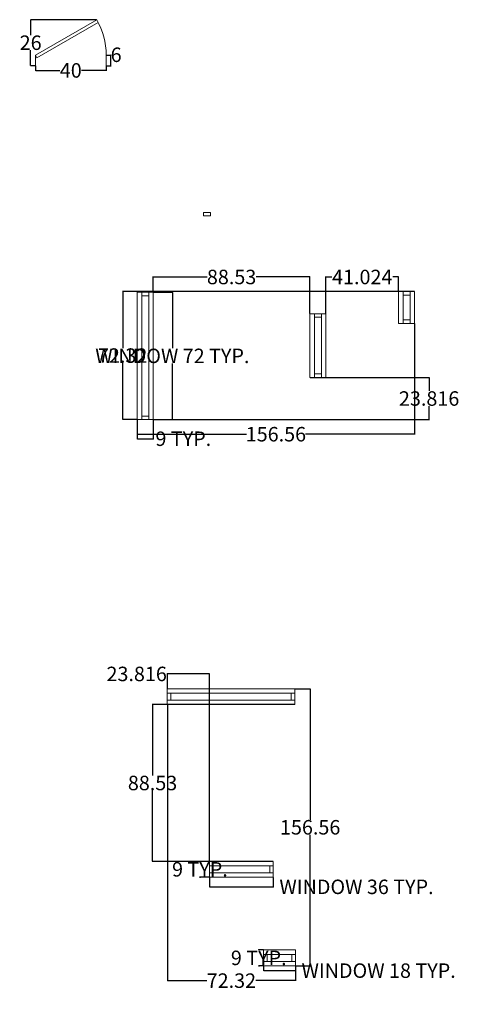
# Model space of a CAD drawing. Units: inches. Extents: x -254 to 1961, y 86 to 3025.
# Tile 4 of 6: x 580 to 828, y 86 to 642. Entities that reach past the tile are written whole.
import ezdxf

# ---------------------------------------------------------------- set-up
doc = ezdxf.new("R2010")
doc.units = ezdxf.units.IN
doc.header["$MEASUREMENT"] = 0
for name, color, linetype, lineweight in [('A-ANNO-DIMS', 2, 'Continuous', 18), ('DOORS', 40, 'Continuous', 18), ('WINDOWS', 50, 'Continuous', 18)]:
    doc.layers.add(name, color=color, linetype=linetype, lineweight=lineweight)
doc.styles.get("Standard").update_dxf_attribs({"font": 'arial.ttf'})
doc.dimstyles.get("Standard").update_dxf_attribs({"dimtxt": 8.18, "dimasz": 0.18, "dimexe": 0.18, "dimexo": 0.0625, "dimgap": 0.09, "dimtad": 0, "dimtih": 1, "dimtoh": 1, "dimdec": 1, "dimzin": 0, "dimdsep": 46, "dimlunit": 3, "dimtxsty": 'Standard', "dimcen": 0.09, "dimadec": 0, "dimazin": 0, "dimtfac": 1, "dimtdec": 1, "dimtofl": 0, "dimtmove": 0, "dimatfit": 3, "dimfxl": 1, "dimtolj": 1, "dimtzin": 0, "dimarcsym": 0})

# ---------------------------------------------------------------- blocks, each defined once
blk = doc.blocks.new('*U2')
for p, q in [((0, 0), (0, -6)), ((40, 0), (40, -6))]:
    blk.add_line(p, q)
blk.add_lwpolyline([(0, 0), (34.64, 20), (35.52, 18.48), (0.87, -1.52)], close=True)
blk.add_arc((0, 0), 40, 0, 30)
blk = doc.blocks.new('WIN-36IN')
for p, q in [((2.5, 35), (2.5, 2)), ((6.5, 35), (6.5, 2))]:
    blk.add_line(p, q)
for points in [[(0, 36), (9, 36), (9, 0), (0, 0)], [(2.5, 36), (6.5, 36), (6.5, 34), (2.5, 34)], [(2.5, 0), (6.5, 0), (6.5, 2), (2.5, 2)]]:
    blk.add_lwpolyline(points, close=True)
blk = doc.blocks.new('WIN-72IN')
for p, q in [((2.5, 70), (2.5, 2)), ((6.5, 70), (6.5, 2))]:
    blk.add_line(p, q)
for points in [[(0, 72), (9, 72), (9, 0), (0, 0)], [(2.5, 72), (6.5, 72), (6.5, 70), (2.5, 70)], [(2.5, 0), (6.5, 0), (6.5, 2), (2.5, 2)]]:
    blk.add_lwpolyline(points, close=True)
blk = doc.blocks.new('WIN-18IN')
for p, q in [((2.5, 16), (2.5, 2)), ((6.5, 16), (6.5, 2))]:
    blk.add_line(p, q)
for points in [[(0, 18), (9, 18), (9, 0), (0, 0)], [(2.5, 18), (6.5, 18), (6.5, 16), (2.5, 16)], [(2.5, 0), (6.5, 0), (6.5, 2), (2.5, 2)]]:
    blk.add_lwpolyline(points, close=True)
blk = doc.blocks.new('*D14')
at = {"layer": 'A-ANNO-DIMS', "color": 0, "lineweight": -2, "transparency": 16777216}
for p, q in [((655.23, 487.85), (666.15, 487.85)), ((665.97, 487.67), (665.97, 456.17)), ((665.97, 416.03), (665.97, 447.53)), ((655.23, 415.85), (666.15, 415.85))]:
    blk.add_line(p, q, dxfattribs=at)
at = {"layer": 'A-ANNO-DIMS', "color": 0, "transparency": 16777216}
for points in [[(665.94, 487.67), (666, 487.67), (665.97, 487.85)], [(665.94, 416.03), (666, 416.03), (665.97, 415.85)]]:
    blk.add_solid(points, dxfattribs=at)
at = {"layer": 'Defpoints', "color": 0, "transparency": 16777216}
for p in [(655.17, 487.85), (665.97, 487.85), (655.17, 415.85)]:
    blk.add_point(p, dxfattribs=at)
at = {"layer": 'A-ANNO-DIMS', "color": 0, "transparency": 16777216, "insert": (665.97, 451.85), "char_height": 8.18, "attachment_point": 5}
blk.add_mtext('\\A1;WINDOW 72 TYP.', dxfattribs=at)
blk = doc.blocks.new('*D15')
at = {"layer": 'A-ANNO-DIMS', "color": 0, "lineweight": -2, "transparency": 16777216}
for p, q in [((646.17, 415.79), (646.17, 404.87)), ((655.17, 415.79), (655.17, 404.87)), ((646.35, 405.05), (654.99, 405.05)), ((655.17, 405.05), (655.35, 405.05))]:
    blk.add_line(p, q, dxfattribs=at)
at = {"layer": 'A-ANNO-DIMS', "color": 0, "transparency": 16777216}
for points in [[(646.35, 405.08), (646.35, 405.02), (646.17, 405.05)], [(654.99, 405.08), (654.99, 405.02), (655.17, 405.05)]]:
    blk.add_solid(points, dxfattribs=at)
at = {"layer": 'Defpoints', "color": 0, "transparency": 16777216}
for p in [(646.17, 415.85), (655.17, 415.85), (655.17, 405.05)]:
    blk.add_point(p, dxfattribs=at)
at = {"layer": 'A-ANNO-DIMS', "color": 0, "transparency": 16777216, "insert": (672.17, 405.05), "char_height": 8.18, "attachment_point": 5}
blk.add_mtext('\\A1;9 TYP.', dxfattribs=at)
blk = doc.blocks.new('*D16')
at = {"layer": 'A-ANNO-DIMS', "color": 0, "lineweight": -2, "transparency": 16777216}
for p, q in [((686.95, 157.24), (686.95, 151.73)), ((722.95, 157.24), (722.95, 151.73)), ((687.13, 151.91), (722.77, 151.91)), ((722.95, 151.91), (723.13, 151.91))]:
    blk.add_line(p, q, dxfattribs=at)
at = {"layer": 'A-ANNO-DIMS', "color": 0, "transparency": 16777216}
for points in [[(687.13, 151.94), (687.13, 151.88), (686.95, 151.91)], [(722.77, 151.94), (722.77, 151.88), (722.95, 151.91)]]:
    blk.add_solid(points, dxfattribs=at)
at = {"layer": 'Defpoints', "color": 0, "transparency": 16777216}
for p in [(686.95, 157.31), (722.95, 157.31), (722.95, 151.91)]:
    blk.add_point(p, dxfattribs=at)
at = {"layer": 'A-ANNO-DIMS', "color": 0, "transparency": 16777216, "insert": (769.96, 151.91), "char_height": 8.18, "attachment_point": 5}
blk.add_mtext('\\A1;WINDOW 36 TYP.', dxfattribs=at)
blk = doc.blocks.new('*D17')
at = {"layer": 'A-ANNO-DIMS', "color": 0, "lineweight": -2, "transparency": 16777216}
for p, q in [((686.89, 166.31), (681.37, 166.31)), ((681.55, 166.49), (681.55, 166.67)), ((686.89, 157.31), (681.37, 157.31)), ((681.55, 157.13), (681.55, 156.95))]:
    blk.add_line(p, q, dxfattribs=at)
at = {"layer": 'A-ANNO-DIMS', "color": 0, "transparency": 16777216}
for points in [[(681.52, 166.49), (681.58, 166.49), (681.55, 166.31)], [(681.52, 157.13), (681.58, 157.13), (681.55, 157.31)]]:
    blk.add_solid(points, dxfattribs=at)
at = {"layer": 'Defpoints', "color": 0, "transparency": 16777216}
for p in [(686.95, 166.31), (681.55, 157.31), (686.95, 157.31)]:
    blk.add_point(p, dxfattribs=at)
at = {"layer": 'A-ANNO-DIMS', "color": 0, "transparency": 16777216, "insert": (681.55, 161.81), "char_height": 8.18, "attachment_point": 5}
blk.add_mtext('\\A1;9 TYP.', dxfattribs=at)
blk = doc.blocks.new('*D18')
at = {"layer": 'A-ANNO-DIMS', "color": 0, "lineweight": -2, "transparency": 16777216}
for p, q in [((717.45, 107.22), (717.45, 104.4)), ((735.45, 107.22), (735.45, 104.4)), ((717.63, 104.58), (735.27, 104.58)), ((735.45, 104.58), (735.63, 104.58))]:
    blk.add_line(p, q, dxfattribs=at)
at = {"layer": 'A-ANNO-DIMS', "color": 0, "transparency": 16777216}
for points in [[(717.63, 104.61), (717.63, 104.55), (717.45, 104.58)], [(735.27, 104.61), (735.27, 104.55), (735.45, 104.58)]]:
    blk.add_solid(points, dxfattribs=at)
at = {"layer": 'Defpoints', "color": 0, "transparency": 16777216}
for p in [(717.45, 107.28), (735.45, 107.28), (735.45, 104.58)]:
    blk.add_point(p, dxfattribs=at)
at = {"layer": 'A-ANNO-DIMS', "color": 0, "transparency": 16777216, "insert": (782.46, 104.58), "char_height": 8.18, "attachment_point": 5}
blk.add_mtext('\\A1;WINDOW 18 TYP.', dxfattribs=at)
blk = doc.blocks.new('*D19')
at = {"layer": 'A-ANNO-DIMS', "color": 0, "lineweight": -2, "transparency": 16777216}
for p, q in [((717.39, 116.28), (714.57, 116.28)), ((714.75, 116.46), (714.75, 116.64)), ((717.39, 107.28), (714.57, 107.28)), ((714.75, 107.1), (714.75, 106.92))]:
    blk.add_line(p, q, dxfattribs=at)
at = {"layer": 'A-ANNO-DIMS', "color": 0, "transparency": 16777216}
for points in [[(714.72, 116.46), (714.78, 116.46), (714.75, 116.28)], [(714.72, 107.1), (714.78, 107.1), (714.75, 107.28)]]:
    blk.add_solid(points, dxfattribs=at)
at = {"layer": 'Defpoints', "color": 0, "transparency": 16777216}
for p in [(717.45, 116.28), (714.75, 107.28), (717.45, 107.28)]:
    blk.add_point(p, dxfattribs=at)
at = {"layer": 'A-ANNO-DIMS', "color": 0, "transparency": 16777216, "insert": (714.75, 111.78), "char_height": 8.18, "attachment_point": 5}
blk.add_mtext('\\A1;9 TYP.', dxfattribs=at)
blk = doc.blocks.new('*D58')
at = {"layer": 'A-ANNO-DIMS', "color": 0, "lineweight": -2, "transparency": 16777216}
for p, q in [((802.72, 470.11), (802.72, 407.42)), ((646.17, 415.79), (646.17, 407.42)), ((646.35, 407.6), (707.76, 407.6)), ((802.54, 407.6), (741.13, 407.6))]:
    blk.add_line(p, q, dxfattribs=at)
at = {"layer": 'A-ANNO-DIMS', "color": 0, "transparency": 16777216}
for points in [[(646.35, 407.63), (646.35, 407.57), (646.17, 407.6)], [(802.54, 407.63), (802.54, 407.57), (802.72, 407.6)]]:
    blk.add_solid(points, dxfattribs=at)
at = {"layer": 'Defpoints', "color": 0, "transparency": 16777216}
for p in [(802.72, 470.17), (646.17, 415.85), (802.72, 407.6)]:
    blk.add_point(p, dxfattribs=at)
at = {"layer": 'A-ANNO-DIMS', "color": 0, "transparency": 16777216, "insert": (724.45, 407.6), "char_height": 8.18, "attachment_point": 5}
blk.add_mtext('\\A1;156.56', dxfattribs=at)
blk = doc.blocks.new('*D59')
at = {"layer": 'A-ANNO-DIMS', "color": 0, "lineweight": -2, "transparency": 16777216}
for p, q in [((802.66, 488.17), (637.74, 488.17)), ((637.92, 487.99), (637.92, 456.28)), ((637.92, 416.03), (637.92, 447.74)), ((646.1, 415.85), (637.74, 415.85))]:
    blk.add_line(p, q, dxfattribs=at)
at = {"layer": 'A-ANNO-DIMS', "color": 0, "transparency": 16777216}
for points in [[(637.89, 487.99), (637.95, 487.99), (637.92, 488.17)], [(637.89, 416.03), (637.95, 416.03), (637.92, 415.85)]]:
    blk.add_solid(points, dxfattribs=at)
at = {"layer": 'Defpoints', "color": 0, "transparency": 16777216}
for p in [(637.92, 488.17), (802.72, 488.17), (646.17, 415.85)]:
    blk.add_point(p, dxfattribs=at)
at = {"layer": 'A-ANNO-DIMS', "color": 0, "transparency": 16777216, "insert": (637.92, 452.01), "char_height": 8.18, "attachment_point": 5}
blk.add_mtext('\\A1;72.32', dxfattribs=at)
blk = doc.blocks.new('*D60')
at = {"layer": 'A-ANNO-DIMS', "color": 0, "lineweight": -2, "transparency": 16777216}
for p, q in [((655.17, 487.91), (655.17, 496.6)), ((655.35, 496.42), (685.54, 496.42)), ((743.52, 496.42), (713.33, 496.42)), ((743.7, 475.73), (743.7, 496.6))]:
    blk.add_line(p, q, dxfattribs=at)
at = {"layer": 'A-ANNO-DIMS', "color": 0, "transparency": 16777216}
for points in [[(655.35, 496.45), (655.35, 496.39), (655.17, 496.42)], [(743.52, 496.45), (743.52, 496.39), (743.7, 496.42)]]:
    blk.add_solid(points, dxfattribs=at)
at = {"layer": 'Defpoints', "color": 0, "transparency": 16777216}
for p in [(743.7, 496.42), (655.17, 487.85), (743.7, 475.67)]:
    blk.add_point(p, dxfattribs=at)
at = {"layer": 'A-ANNO-DIMS', "color": 0, "transparency": 16777216, "insert": (699.43, 496.42), "char_height": 8.18, "attachment_point": 5}
blk.add_mtext('\\A1;88.53', dxfattribs=at)
blk = doc.blocks.new('*D61')
at = {"layer": 'A-ANNO-DIMS', "color": 0, "lineweight": -2, "transparency": 16777216}
for p, q in [((752.7, 475.73), (752.7, 496.6)), ((752.88, 496.42), (755.99, 496.42)), ((793.54, 496.42), (790.43, 496.42)), ((793.72, 488.23), (793.72, 496.6))]:
    blk.add_line(p, q, dxfattribs=at)
at = {"layer": 'A-ANNO-DIMS', "color": 0, "transparency": 16777216}
for points in [[(752.88, 496.45), (752.88, 496.39), (752.7, 496.42)], [(793.54, 496.45), (793.54, 496.39), (793.72, 496.42)]]:
    blk.add_solid(points, dxfattribs=at)
at = {"layer": 'Defpoints', "color": 0, "transparency": 16777216}
for p in [(793.72, 496.42), (793.72, 488.17), (752.7, 475.67)]:
    blk.add_point(p, dxfattribs=at)
at = {"layer": 'A-ANNO-DIMS', "color": 0, "transparency": 16777216, "insert": (773.21, 496.42), "char_height": 8.18, "attachment_point": 5}
blk.add_mtext('\\A1;41.024', dxfattribs=at)
blk = doc.blocks.new('*D62')
at = {"layer": 'A-ANNO-DIMS', "color": 0, "lineweight": -2, "transparency": 16777216}
for p, q in [((743.76, 439.67), (811.15, 439.67)), ((810.97, 439.49), (810.97, 432.03)), ((810.97, 416.03), (810.97, 423.49)), ((655.23, 415.85), (811.15, 415.85))]:
    blk.add_line(p, q, dxfattribs=at)
at = {"layer": 'A-ANNO-DIMS', "color": 0, "transparency": 16777216}
for points in [[(810.94, 439.49), (811, 439.49), (810.97, 439.67)], [(810.94, 416.03), (811, 416.03), (810.97, 415.85)]]:
    blk.add_solid(points, dxfattribs=at)
at = {"layer": 'Defpoints', "color": 0, "transparency": 16777216}
for p in [(743.7, 439.67), (810.97, 439.67), (655.17, 415.85)]:
    blk.add_point(p, dxfattribs=at)
at = {"layer": 'A-ANNO-DIMS', "color": 0, "transparency": 16777216, "insert": (810.97, 427.76), "char_height": 8.18, "attachment_point": 5}
blk.add_mtext('\\A1;23.816', dxfattribs=at)
blk = doc.blocks.new('*D63')
at = {"layer": 'A-ANNO-DIMS', "color": 0, "lineweight": -2, "transparency": 16777216}
for p, q in [((735.2, 263.84), (743.98, 263.84)), ((743.8, 263.66), (743.8, 189.83)), ((743.8, 107.46), (743.8, 181.3)), ((735.52, 107.28), (743.98, 107.28))]:
    blk.add_line(p, q, dxfattribs=at)
at = {"layer": 'A-ANNO-DIMS', "color": 0, "transparency": 16777216}
for points in [[(743.77, 263.66), (743.83, 263.66), (743.8, 263.84)], [(743.77, 107.46), (743.83, 107.46), (743.8, 107.28)]]:
    blk.add_solid(points, dxfattribs=at)
at = {"layer": 'Defpoints', "color": 0, "transparency": 16777216}
for p in [(735.14, 263.84), (743.8, 263.84), (735.45, 107.28)]:
    blk.add_point(p, dxfattribs=at)
at = {"layer": 'A-ANNO-DIMS', "color": 0, "transparency": 16777216, "insert": (743.8, 185.56), "char_height": 8.18, "attachment_point": 5}
blk.add_mtext('\\A1;156.56', dxfattribs=at)
blk = doc.blocks.new('*D64')
at = {"layer": 'A-ANNO-DIMS', "color": 0, "lineweight": -2, "transparency": 16777216}
for p, q in [((735.07, 254.84), (654.61, 254.84)), ((654.79, 254.66), (654.79, 214.84)), ((654.79, 166.49), (654.79, 206.3)), ((722.89, 166.31), (654.61, 166.31))]:
    blk.add_line(p, q, dxfattribs=at)
at = {"layer": 'A-ANNO-DIMS', "color": 0, "transparency": 16777216}
for points in [[(654.76, 254.66), (654.82, 254.66), (654.79, 254.84)], [(654.76, 166.49), (654.82, 166.49), (654.79, 166.31)]]:
    blk.add_solid(points, dxfattribs=at)
at = {"layer": 'Defpoints', "color": 0, "transparency": 16777216}
for p in [(735.14, 254.84), (654.79, 166.31), (722.95, 166.31)]:
    blk.add_point(p, dxfattribs=at)
at = {"layer": 'A-ANNO-DIMS', "color": 0, "transparency": 16777216, "insert": (654.79, 210.57), "char_height": 8.18, "attachment_point": 5}
blk.add_mtext('\\A1;88.53', dxfattribs=at)
blk = doc.blocks.new('*D65')
at = {"layer": 'A-ANNO-DIMS', "color": 0, "lineweight": -2, "transparency": 16777216}
for p, q in [((663.14, 272.19), (662.96, 272.19)), ((663.14, 263.9), (663.14, 272.37)), ((686.77, 272.19), (663.32, 272.19)), ((686.95, 166.37), (686.95, 272.37))]:
    blk.add_line(p, q, dxfattribs=at)
at = {"layer": 'A-ANNO-DIMS', "color": 0, "transparency": 16777216}
for points in [[(663.32, 272.22), (663.32, 272.16), (663.14, 272.19)], [(686.77, 272.22), (686.77, 272.16), (686.95, 272.19)]]:
    blk.add_solid(points, dxfattribs=at)
at = {"layer": 'Defpoints', "color": 0, "transparency": 16777216}
for p in [(663.14, 272.19), (663.14, 263.84), (686.95, 166.31)]:
    blk.add_point(p, dxfattribs=at)
at = {"layer": 'A-ANNO-DIMS', "color": 0, "transparency": 16777216, "insert": (645.82, 272.19), "char_height": 8.18, "attachment_point": 5}
blk.add_mtext('\\A1;23.816', dxfattribs=at)
blk = doc.blocks.new('*D66')
at = {"layer": 'A-ANNO-DIMS', "color": 0, "lineweight": -2, "transparency": 16777216}
for p, q in [((663.14, 254.78), (663.14, 98.75)), ((735.45, 107.22), (735.45, 98.75)), ((663.32, 98.93), (685.48, 98.93)), ((735.27, 98.93), (713.11, 98.93))]:
    blk.add_line(p, q, dxfattribs=at)
at = {"layer": 'A-ANNO-DIMS', "color": 0, "transparency": 16777216}
for points in [[(663.32, 98.96), (663.32, 98.9), (663.14, 98.93)], [(735.27, 98.96), (735.27, 98.9), (735.45, 98.93)]]:
    blk.add_solid(points, dxfattribs=at)
at = {"layer": 'Defpoints', "color": 0, "transparency": 16777216}
for p in [(663.14, 254.84), (735.45, 107.28), (735.45, 98.93)]:
    blk.add_point(p, dxfattribs=at)
at = {"layer": 'A-ANNO-DIMS', "color": 0, "transparency": 16777216, "insert": (699.3, 98.93), "char_height": 8.18, "attachment_point": 5}
blk.add_mtext('\\A1;72.32', dxfattribs=at)
blk = doc.blocks.new('*D67')
at = {"layer": 'A-ANNO-DIMS', "color": 0, "lineweight": -2, "transparency": 16777216}
for p, q in [((588.61, 615.69), (588.61, 612.93)), ((588.79, 613.11), (602.51, 613.11)), ((628.43, 613.11), (614.71, 613.11)), ((628.61, 615.69), (628.61, 612.93))]:
    blk.add_line(p, q, dxfattribs=at)
at = {"layer": 'A-ANNO-DIMS', "color": 0, "transparency": 16777216}
for points in [[(588.79, 613.14), (588.79, 613.08), (588.61, 613.11)], [(628.43, 613.14), (628.43, 613.08), (628.61, 613.11)]]:
    blk.add_solid(points, dxfattribs=at)
at = {"layer": 'Defpoints', "color": 0, "transparency": 16777216}
for p in [(588.61, 615.76), (628.61, 615.76), (628.61, 613.11)]:
    blk.add_point(p, dxfattribs=at)
at = {"layer": 'A-ANNO-DIMS', "color": 0, "transparency": 16777216, "insert": (608.61, 613.11), "char_height": 8.18, "attachment_point": 5}
blk.add_mtext('\\A1;40', dxfattribs=at)
blk = doc.blocks.new('*D68')
at = {"layer": 'A-ANNO-DIMS', "color": 0, "lineweight": -2, "transparency": 16777216}
for p, q in [((623.19, 641.76), (585.78, 641.76)), ((585.96, 641.58), (585.96, 633.02)), ((585.96, 615.94), (585.96, 624.49)), ((588.55, 615.76), (585.78, 615.76))]:
    blk.add_line(p, q, dxfattribs=at)
at = {"layer": 'A-ANNO-DIMS', "color": 0, "transparency": 16777216}
for points in [[(585.93, 641.58), (585.99, 641.58), (585.96, 641.76)], [(585.93, 615.94), (585.99, 615.94), (585.96, 615.76)]]:
    blk.add_solid(points, dxfattribs=at)
at = {"layer": 'Defpoints', "color": 0, "transparency": 16777216}
for p in [(585.96, 641.76), (623.25, 641.76), (588.61, 615.76)]:
    blk.add_point(p, dxfattribs=at)
at = {"layer": 'A-ANNO-DIMS', "color": 0, "transparency": 16777216, "insert": (585.96, 628.76), "char_height": 8.18, "attachment_point": 5}
blk.add_mtext('\\A1;26', dxfattribs=at)
blk = doc.blocks.new('*D69')
at = {"layer": 'A-ANNO-DIMS', "color": 0, "lineweight": -2, "transparency": 16777216}
for p, q in [((628.68, 621.76), (631.44, 621.76)), ((631.26, 621.76), (631.26, 621.94)), ((631.26, 621.94), (631.44, 621.94)), ((631.26, 615.94), (631.26, 621.58)), ((628.68, 615.76), (631.44, 615.76))]:
    blk.add_line(p, q, dxfattribs=at)
at = {"layer": 'A-ANNO-DIMS', "color": 0, "transparency": 16777216}
for points in [[(631.23, 621.58), (631.29, 621.58), (631.26, 621.76)], [(631.23, 615.94), (631.29, 615.94), (631.26, 615.76)]]:
    blk.add_solid(points, dxfattribs=at)
at = {"layer": 'Defpoints', "color": 0, "transparency": 16777216}
for p in [(628.61, 621.76), (631.26, 621.76), (628.61, 615.76)]:
    blk.add_point(p, dxfattribs=at)
at = {"layer": 'A-ANNO-DIMS', "color": 0, "transparency": 16777216, "insert": (634.23, 621.94), "char_height": 8.18, "attachment_point": 5}
blk.add_mtext('\\A1;6', dxfattribs=at)

msp = doc.modelspace()

# ---------------------------------------------------------------- linework, layer by layer
at = {"layer": 'WINDOWS'}
msp.add_lwpolyline([(683.4987, 532.8847), (687.4987, 532.8847), (687.4987, 530.8847), (683.4987, 530.8847)], close=True, dxfattribs=at)

# ---------------------------------------------------------------- block references
at = {"layer": 'DOORS'}
msp.add_blockref('*U2', (588.6137, 621.7573), dxfattribs=at)
at = {"layer": 'WINDOWS'}
for name, p in [('WIN-72IN', (646.167, 415.85)), ('WIN-18IN', (793.724, 470.168)), ('WIN-36IN', (743.7, 439.666))]:
    msp.add_blockref(name, p, dxfattribs=at)
for name, p, rotation in [('WIN-72IN', (663.1365, 263.8402), 270.0000000000007), ('WIN-36IN', (686.9525, 166.3072), 269.9999999999991), ('WIN-18IN', (717.4545, 116.2832), 269.9999999999978)]:
    msp.add_blockref(name, p, dxfattribs=dict(at, rotation=rotation))

# ---------------------------------------------------------------- dimensions: what is measured, and where the dimension line sits
at = {"layer": 'A-ANNO-DIMS'}
for base, p1, p2, override, picture, middle in [((585.9637, 641.7573), (588.6137, 615.7573), (623.2547, 641.7573), {"dimdec": 0, "dimlfac": 1, "dimrnd": 0, "dimzin": 0, "dimdsep": 46, "dimlunit": 2}, '*D68', (585.9637, 628.7573)), ((631.2637, 621.7573), (628.6137, 615.7573), (628.6137, 621.7573), {"dimdec": 0, "dimlfac": 1, "dimrnd": 0, "dimzin": 0, "dimdsep": 46, "dimlunit": 2}, '*D69', (634.2343, 621.9373)), ((637.9171, 488.168), (646.1671, 415.8499), (802.7242, 488.168), {"dimdec": 2, "dimlfac": 1, "dimrnd": 0, "dimzin": 0, "dimdsep": 46, "dimlunit": 2}, '*D59', (637.9171, 452.009)), ((810.9742, 439.6661), (655.1671, 415.8499), (743.7, 439.6661), {"dimdec": 3, "dimlfac": 1, "dimrnd": 0, "dimzin": 0, "dimdsep": 46, "dimlunit": 2}, '*D62', (810.9742, 427.758)), ((743.8045, 263.8401), (735.4545, 107.2831), (735.1365, 263.8401), {"dimdec": 2, "dimlfac": 1, "dimrnd": 0, "dimzin": 0, "dimdsep": 46, "dimlunit": 2}, '*D63', (743.8045, 185.5616)), ((654.7865, 166.3073), (735.1365, 254.8401), (722.9526, 166.3073), {"dimdec": 2, "dimlfac": 1, "dimrnd": 0, "dimzin": 0, "dimdsep": 46, "dimlunit": 2}, '*D64', (654.7865, 210.5737))]:
    dim = msp.add_linear_dim(base=base, p1=p1, p2=p2, angle=90, dimstyle='Standard', override=override, dxfattribs=at)
    dim.commit()
    dim.dimension.update_dxf_attribs({"geometry": picture, "text_midpoint": middle})
for base, p1, p2, override, picture, middle in [((628.6137, 613.1073), (588.6137, 615.7573), (628.6137, 615.7573), {"dimdec": 0, "dimlfac": 1, "dimrnd": 0, "dimzin": 0, "dimdsep": 46, "dimlunit": 2}, '*D67', (608.6137, 613.1073)), ((743.7, 496.418), (655.1671, 487.8499), (743.7, 475.6661), {"dimdec": 2, "dimlfac": 1, "dimrnd": 0, "dimzin": 0, "dimdsep": 46, "dimlunit": 2}, '*D60', (699.4335, 496.418)), ((793.7242, 496.418), (752.7, 475.6661), (793.7242, 488.168), {"dimdec": 3, "dimlfac": 1, "dimrnd": 0, "dimzin": 0, "dimdsep": 46, "dimlunit": 2}, '*D61', (773.2121, 496.418)), ((802.7242, 407.5999), (646.1671, 415.8499), (802.7242, 470.168), {"dimdec": 2, "dimlfac": 1, "dimrnd": 0, "dimzin": 0, "dimdsep": 46, "dimlunit": 2}, '*D58', (724.4457, 407.5999)), ((663.1365, 272.1901), (686.9526, 166.3073), (663.1365, 263.8401), {"dimdec": 3, "dimlfac": 1, "dimrnd": 0, "dimzin": 0, "dimdsep": 46, "dimlunit": 2}, '*D65', (645.8201, 272.1901)), ((735.4545, 98.9331), (663.1365, 254.8401), (735.4545, 107.2831), {"dimdec": 2, "dimlfac": 1, "dimrnd": 0, "dimzin": 0, "dimdsep": 46, "dimlunit": 2}, '*D66', (699.2955, 98.9331))]:
    dim = msp.add_linear_dim(base=base, p1=p1, p2=p2, dimstyle='Standard', override=override, dxfattribs=at)
    dim.commit()
    dim.dimension.update_dxf_attribs({"geometry": picture, "text_midpoint": middle})
for base, p1, p2, angle, text, picture, middle in [((665.9671, 487.8499), (655.1671, 415.8499), (655.1671, 487.8499), 90, 'WINDOW <> TYP.', '*D14', (665.9671, 451.8499)), ((681.5526, 157.3073), (686.9526, 166.3073), (686.9526, 157.3073), 270, '<> TYP.', '*D17', (681.5526, 161.8073)), ((714.7545, 107.2831), (717.4545, 116.2831), (717.4545, 107.2831), 270, '<> TYP.', '*D19', (714.7545, 111.7831))]:
    dim = msp.add_linear_dim(base=base, p1=p1, p2=p2, angle=angle, text=text, dimstyle='Standard', override={"dimdec": 0, "dimlfac": 1, "dimrnd": 0, "dimzin": 0, "dimdsep": 46, "dimlunit": 2}, dxfattribs=at)
    dim.commit()
    dim.dimension.update_dxf_attribs({"geometry": picture, "text_midpoint": middle})
for base, p1, p2, text, picture, middle in [((655.1671, 405.0499), (646.1671, 415.8499), (655.1671, 415.8499), '<> TYP.', '*D15', (672.1682, 405.0499)), ((722.9526, 151.9073), (686.9526, 157.3073), (722.9526, 157.3073), 'WINDOW <> TYP.', '*D16', (769.9563, 151.9073)), ((735.4545, 104.5831), (717.4545, 107.2831), (735.4545, 107.2831), 'WINDOW <> TYP.', '*D18', (782.4582, 104.5831))]:
    dim = msp.add_linear_dim(base=base, p1=p1, p2=p2, text=text, dimstyle='Standard', override={"dimdec": 0, "dimlfac": 1, "dimrnd": 0, "dimzin": 0, "dimdsep": 46, "dimlunit": 2}, dxfattribs=at)
    dim.commit()
    dim.dimension.update_dxf_attribs({"geometry": picture, "text_midpoint": middle})

doc.saveas('drawing.dxf')
